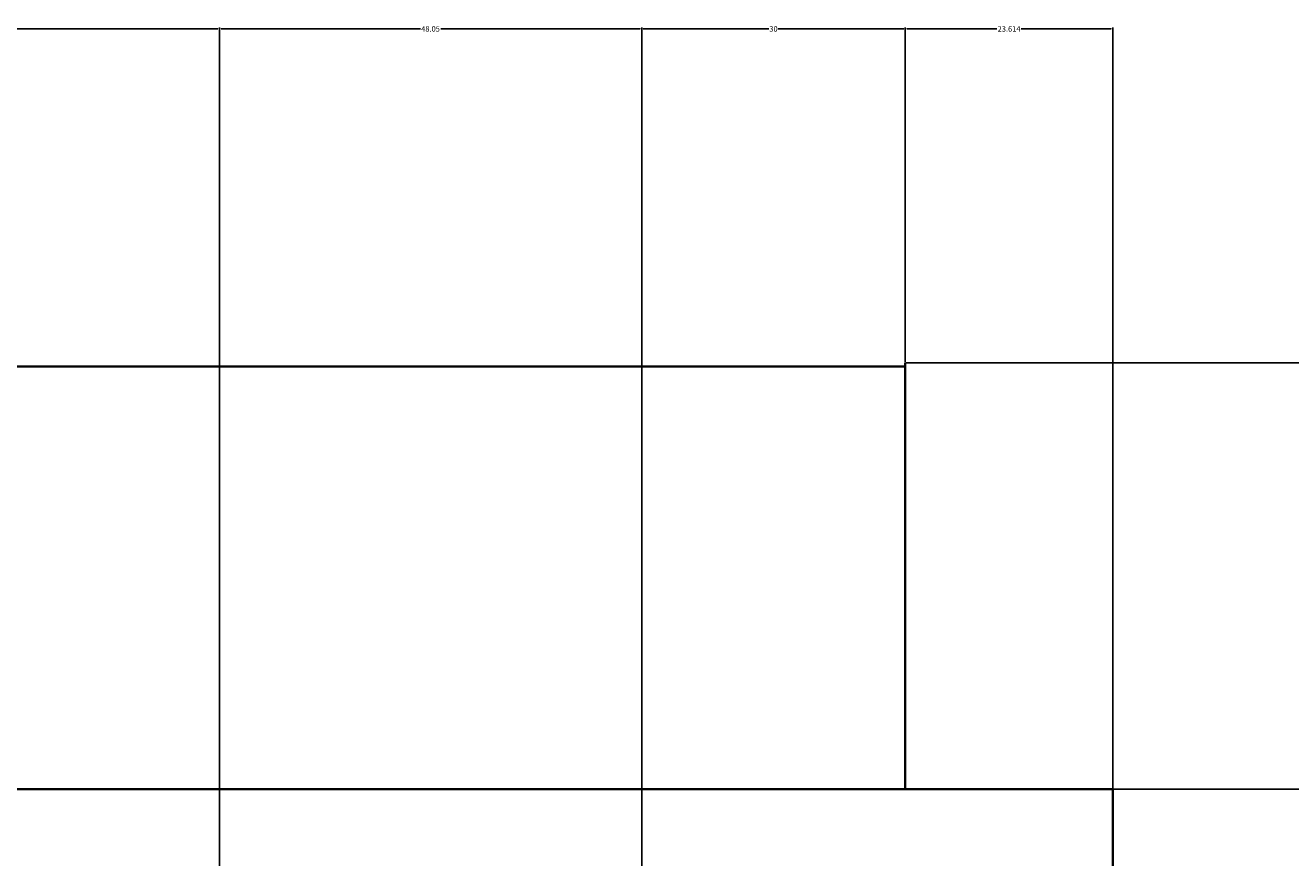
# Model space of a CAD drawing. Units: inches. Extents: x -13 to 809, y 112 to 656.
# Tile 54 of 55: x 521 to 665, y 561 to 656. Entities that reach past the tile are written whole.
import ezdxf

# ---------------------------------------------------------------- set-up
doc = ezdxf.new("R2010")
doc.units = ezdxf.units.IN
doc.header["$MEASUREMENT"] = 0
doc.layers.add('A-ANNO-DIMS', color=2, linetype='Continuous', lineweight=18)
doc.layers.add('A-ELEV', color=7, linetype='Continuous', lineweight=35)
doc.styles.get("Standard").update_dxf_attribs({"font": 'arial.ttf'})
doc.dimstyles.get("Standard").update_dxf_attribs({"dimtxt": 0.625, "dimasz": 0.18, "dimexe": 0.18, "dimexo": 0.0625, "dimgap": 0.09, "dimtad": 0, "dimtih": 1, "dimtoh": 1, "dimdec": 4, "dimzin": 0, "dimdsep": 46, "dimlunit": 4, "dimtxsty": 'Standard', "dimcen": 0.09, "dimadec": 0, "dimazin": 0, "dimtfac": 1, "dimtdec": 4, "dimtofl": 0, "dimtmove": 0, "dimatfit": 3, "dimfxl": 1, "dimtolj": 1, "dimtzin": 0, "dimarcsym": 0})

# ---------------------------------------------------------------- blocks, each defined once
blk = doc.blocks.new('*D27')
at = {"layer": 'A-ANNO-DIMS', "color": 0, "lineweight": -2, "transparency": 16777216}
for p, q in [((471.1, 470.94), (471.1, 655.96)), ((471.28, 655.78), (505.89, 655.78)), ((542.78, 655.78), (508.17, 655.78)), ((542.96, 524.34), (542.96, 655.96))]:
    blk.add_line(p, q, dxfattribs=at)
at = {"layer": 'A-ANNO-DIMS', "color": 0, "transparency": 16777216}
for points in [[(471.28, 655.81), (471.28, 655.75), (471.1, 655.78)], [(542.78, 655.81), (542.78, 655.75), (542.96, 655.78)]]:
    blk.add_solid(points, dxfattribs=at)
at = {"layer": 'Defpoints', "color": 0, "transparency": 16777216}
for p in [(542.96, 655.78), (542.96, 524.28), (471.1, 470.88)]:
    blk.add_point(p, dxfattribs=at)
at = {"layer": 'A-ANNO-DIMS', "color": 0, "transparency": 16777216, "insert": (507.03, 655.78), "char_height": 0.625, "attachment_point": 5}
blk.add_mtext('\\A1;71.86', dxfattribs=at)
blk = doc.blocks.new('*D28')
at = {"layer": 'A-ANNO-DIMS', "color": 0, "lineweight": -2, "transparency": 16777216}
for p, q in [((542.96, 524.34), (542.96, 655.96)), ((543.14, 655.78), (565.83, 655.78)), ((590.83, 655.78), (568.14, 655.78)), ((591.01, 558.58), (591.01, 655.96))]:
    blk.add_line(p, q, dxfattribs=at)
at = {"layer": 'A-ANNO-DIMS', "color": 0, "transparency": 16777216}
for points in [[(543.14, 655.81), (543.14, 655.75), (542.96, 655.78)], [(590.83, 655.81), (590.83, 655.75), (591.01, 655.78)]]:
    blk.add_solid(points, dxfattribs=at)
at = {"layer": 'Defpoints', "color": 0, "transparency": 16777216}
for p in [(591.01, 655.78), (591.01, 558.52), (542.96, 524.28)]:
    blk.add_point(p, dxfattribs=at)
at = {"layer": 'A-ANNO-DIMS', "color": 0, "transparency": 16777216, "insert": (566.98, 655.78), "char_height": 0.625, "attachment_point": 5}
blk.add_mtext('\\A1;48.05', dxfattribs=at)
blk = doc.blocks.new('*D29')
at = {"layer": 'A-ANNO-DIMS', "color": 0, "lineweight": -2, "transparency": 16777216}
for p, q in [((591.01, 558.58), (591.01, 655.96)), ((591.19, 655.78), (605.47, 655.78)), ((620.83, 655.78), (606.54, 655.78)), ((621.01, 617.85), (621.01, 655.96))]:
    blk.add_line(p, q, dxfattribs=at)
at = {"layer": 'A-ANNO-DIMS', "color": 0, "transparency": 16777216}
for points in [[(591.19, 655.81), (591.19, 655.75), (591.01, 655.78)], [(620.83, 655.81), (620.83, 655.75), (621.01, 655.78)]]:
    blk.add_solid(points, dxfattribs=at)
at = {"layer": 'Defpoints', "color": 0, "transparency": 16777216}
for p in [(621.01, 655.78), (621.01, 617.78), (591.01, 558.52)]:
    blk.add_point(p, dxfattribs=at)
at = {"layer": 'A-ANNO-DIMS', "color": 0, "transparency": 16777216, "insert": (606.01, 655.78), "char_height": 0.625, "attachment_point": 5}
blk.add_mtext('\\A1;30', dxfattribs=at)
blk = doc.blocks.new('*D30')
at = {"layer": 'A-ANNO-DIMS', "color": 0, "lineweight": -2, "transparency": 16777216}
for p, q in [((621.01, 617.85), (621.01, 655.96)), ((621.19, 655.78), (631.42, 655.78)), ((644.44, 655.78), (634.21, 655.78)), ((644.62, 569.3), (644.62, 655.96))]:
    blk.add_line(p, q, dxfattribs=at)
at = {"layer": 'A-ANNO-DIMS', "color": 0, "transparency": 16777216}
for points in [[(621.19, 655.81), (621.19, 655.75), (621.01, 655.78)], [(644.44, 655.81), (644.44, 655.75), (644.62, 655.78)]]:
    blk.add_solid(points, dxfattribs=at)
at = {"layer": 'Defpoints', "color": 0, "transparency": 16777216}
for p in [(644.62, 655.78), (621.01, 617.78), (644.62, 569.24)]:
    blk.add_point(p, dxfattribs=at)
at = {"layer": 'A-ANNO-DIMS', "color": 0, "transparency": 16777216, "insert": (632.82, 655.78), "char_height": 0.625, "attachment_point": 5}
blk.add_mtext('\\A1;23.614', dxfattribs=at)
blk = doc.blocks.new('*D31')
at = {"layer": 'A-ANNO-DIMS', "color": 0, "lineweight": -2, "transparency": 16777216}
for p, q in [((621.07, 617.78), (807.77, 617.78)), ((807.59, 617.6), (807.59, 384.56)), ((807.59, 150.7), (807.59, 383.74)), ((621.07, 150.52), (807.77, 150.52))]:
    blk.add_line(p, q, dxfattribs=at)
at = {"layer": 'A-ANNO-DIMS', "color": 0, "transparency": 16777216}
for points in [[(807.56, 617.6), (807.62, 617.6), (807.59, 617.78)], [(807.56, 150.7), (807.62, 150.7), (807.59, 150.52)]]:
    blk.add_solid(points, dxfattribs=at)
at = {"layer": 'Defpoints', "color": 0, "transparency": 16777216}
for p in [(621.01, 617.78), (807.59, 617.78), (621.01, 150.52)]:
    blk.add_point(p, dxfattribs=at)
at = {"layer": 'A-ANNO-DIMS', "color": 0, "transparency": 16777216, "insert": (807.59, 384.15), "char_height": 0.625, "attachment_point": 5}
blk.add_mtext('\\A1;467.3', dxfattribs=at)
blk = doc.blocks.new('*D38')
at = {"layer": 'A-ANNO-DIMS', "color": 0, "lineweight": -2, "transparency": 16777216}
for p, q in [((644.68, 569.24), (807.77, 569.24)), ((807.59, 569.06), (807.59, 564.29)), ((807.59, 558.7), (807.59, 563.47)), ((644.68, 558.52), (807.77, 558.52))]:
    blk.add_line(p, q, dxfattribs=at)
at = {"layer": 'A-ANNO-DIMS', "color": 0, "transparency": 16777216}
for points in [[(807.56, 569.06), (807.62, 569.06), (807.59, 569.24)], [(807.56, 558.7), (807.62, 558.7), (807.59, 558.52)]]:
    blk.add_solid(points, dxfattribs=at)
at = {"layer": 'Defpoints', "color": 0, "transparency": 16777216}
for p in [(644.62, 569.24), (807.59, 569.24), (644.62, 558.52)]:
    blk.add_point(p, dxfattribs=at)
at = {"layer": 'A-ANNO-DIMS', "color": 0, "transparency": 16777216, "insert": (807.59, 563.88), "char_height": 0.625, "attachment_point": 5}
blk.add_mtext('\\A1;10.721', dxfattribs=at)

msp = doc.modelspace()

# ---------------------------------------------------------------- linework, layer by layer
at = {"layer": 'A-ELEV'}
for p, q in [((311.6991, 617.3708), (621.008, 617.3708)), ((621.008, 569.2414), (621.008, 617.7828)), ((292.923, 569.2414), (644.6221, 569.2414)), ((644.6221, 569.2414), (644.6221, 558.5199))]:
    msp.add_line(p, q, dxfattribs=at)

# ---------------------------------------------------------------- dimensions: what is measured, and where the dimension line sits
at = {"layer": 'A-ANNO-DIMS'}
for base, p1, p2, override, picture, middle in [((542.9617, 655.7828), (471.0998, 470.8765), (542.9617, 524.281), {"dimdec": 2, "dimlfac": 1, "dimrnd": 0, "dimzin": 0, "dimdsep": 46, "dimlunit": 2}, '*D27', (507.0308, 655.7828)), ((591.008, 655.7828), (542.9617, 524.281), (591.008, 558.5199), {"dimdec": 2, "dimlfac": 1, "dimrnd": 0, "dimzin": 0, "dimdsep": 46, "dimlunit": 2}, '*D28', (566.9849, 655.7828)), ((621.008, 655.7828), (591.008, 558.5199), (621.008, 617.7828), {"dimdec": 0, "dimlfac": 1, "dimrnd": 0, "dimzin": 0, "dimdsep": 46, "dimlunit": 2}, '*D29', (606.008, 655.7828)), ((644.6221, 655.7828), (621.008, 617.7828), (644.6221, 569.2414), {"dimdec": 3, "dimlfac": 1, "dimrnd": 0, "dimzin": 0, "dimdsep": 46, "dimlunit": 2}, '*D30', (632.8151, 655.7828))]:
    dim = msp.add_linear_dim(base=base, p1=p1, p2=p2, dimstyle='Standard', override=override, dxfattribs=at)
    dim.commit()
    dim.dimension.update_dxf_attribs({"geometry": picture, "text_midpoint": middle})
for base, p1, p2, override, picture, middle in [((807.5888, 617.7828), (621.008, 150.5199), (621.008, 617.7828), {"dimdec": 1, "dimlfac": 1, "dimrnd": 0, "dimzin": 0, "dimdsep": 46, "dimlunit": 2}, '*D31', (807.5888, 384.1514)), ((807.588831, 569.241385), (644.622094, 558.519894), (644.622094, 569.241385), {"dimdec": 3, "dimlfac": 1, "dimrnd": 0, "dimzin": 0, "dimdsep": 46, "dimlunit": 2}, '*D38', (807.588831, 563.88064))]:
    dim = msp.add_linear_dim(base=base, p1=p1, p2=p2, angle=90, dimstyle='Standard', override=override, dxfattribs=at)
    dim.commit()
    dim.dimension.update_dxf_attribs({"geometry": picture, "text_midpoint": middle})

doc.saveas('drawing.dxf')
